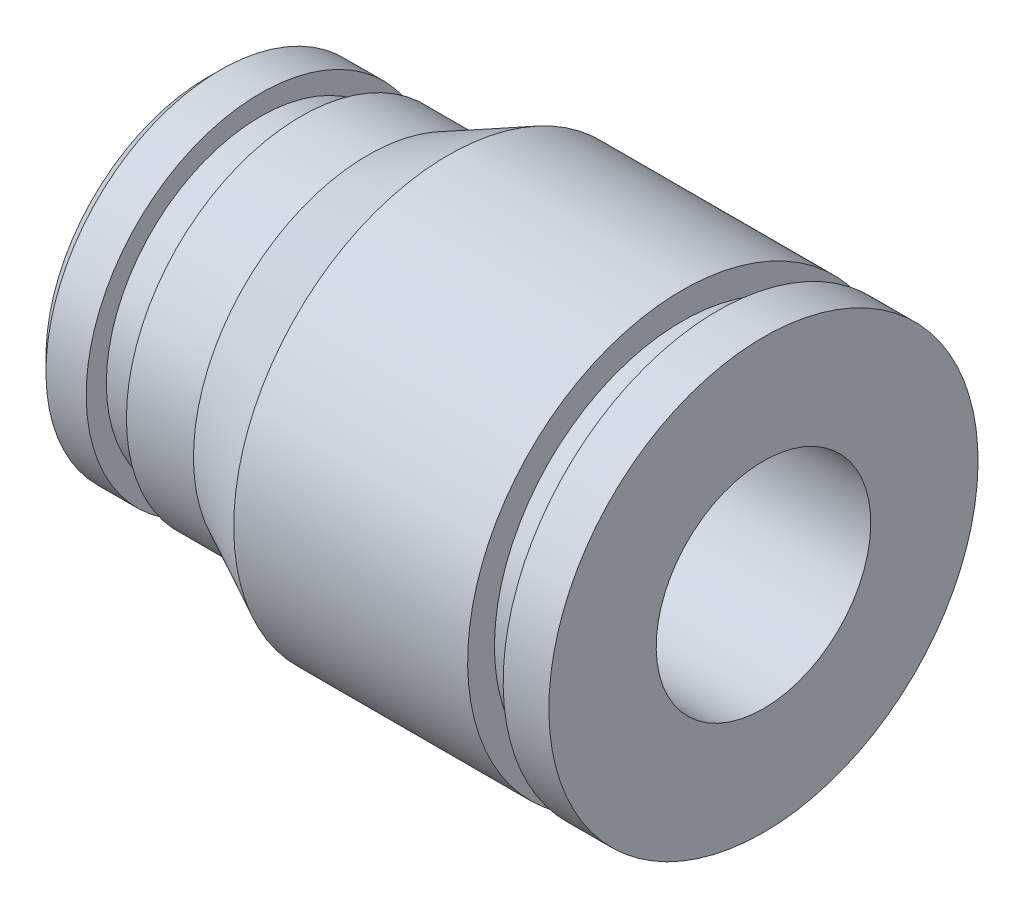
ISO-10303-21;
HEADER;
FILE_DESCRIPTION(('STEP AP214'),'2;1');
FILE_NAME('part.step','',(''),(''),'','','');
FILE_SCHEMA(('AUTOMOTIVE_DESIGN { 1 0 10303 214 1 1 1 1 }'));
ENDSEC;
DATA;
#1=APPLICATION_CONTEXT('core data for automotive mechanical design processes');
#2=APPLICATION_PROTOCOL_DEFINITION('international standard','automotive_design',2000,#1);
#3=PRODUCT_CONTEXT('',#1,'mechanical');
#4=PRODUCT('Part','Part','',(#3));
#5=PRODUCT_RELATED_PRODUCT_CATEGORY('part','',(#4));
#6=PRODUCT_DEFINITION_FORMATION('','',#4);
#7=PRODUCT_DEFINITION_CONTEXT('part definition',#1,'design');
#8=PRODUCT_DEFINITION('design','',#6,#7);
#9=PRODUCT_DEFINITION_SHAPE('','',#8);
#10=(LENGTH_UNIT() NAMED_UNIT(*) SI_UNIT(.MILLI.,.METRE.));
#11=(NAMED_UNIT(*) PLANE_ANGLE_UNIT() SI_UNIT($,.RADIAN.));
#12=(NAMED_UNIT(*) SI_UNIT($,.STERADIAN.) SOLID_ANGLE_UNIT());
#13=UNCERTAINTY_MEASURE_WITH_UNIT(LENGTH_MEASURE(1.E-05),#10,'distance_accuracy_value','');
#14=(GEOMETRIC_REPRESENTATION_CONTEXT(3) GLOBAL_UNCERTAINTY_ASSIGNED_CONTEXT((#13)) GLOBAL_UNIT_ASSIGNED_CONTEXT((#10,
#11,#12)) REPRESENTATION_CONTEXT('',''));
#15=CARTESIAN_POINT('',(0.,0.,0.));
#16=DIRECTION('',(0.,0.,1.));
#17=DIRECTION('',(1.,0.,0.));
#18=AXIS2_PLACEMENT_3D('',#15,#16,#17);
#19=CARTESIAN_POINT('',(-43.7918179780591,0.,0.));
#20=DIRECTION('',(-1.,0.,0.));
#21=DIRECTION('',(0.,-1.,0.));
#22=AXIS2_PLACEMENT_3D('',#19,#20,#21);
#23=CYLINDRICAL_SURFACE('',#22,13.);
#24=CARTESIAN_POINT('',(-8.5973527361911,0.,0.));
#25=DIRECTION('',(-1.,0.,0.));
#26=DIRECTION('',(0.,-1.,0.));
#27=AXIS2_PLACEMENT_3D('',#24,#25,#26);
#28=CIRCLE('',#27,13.);
#29=CARTESIAN_POINT('',(-8.59735273619109,-13.,0.));
#30=VERTEX_POINT('',#29);
#31=EDGE_CURVE('E76',#30,#30,#28,.T.);
#32=ORIENTED_EDGE('',*,*,#31,.F.);
#33=EDGE_LOOP('',(#32));
#34=FACE_BOUND('',#33,.T.);
#35=CARTESIAN_POINT('',(-5.59735273619109,0.,0.));
#36=DIRECTION('',(1.,0.,0.));
#37=DIRECTION('',(0.,0.,-1.));
#38=AXIS2_PLACEMENT_3D('',#35,#36,#37);
#39=CIRCLE('',#38,13.);
#40=CARTESIAN_POINT('',(-5.59735273619109,0.,-13.));
#41=VERTEX_POINT('',#40);
#42=EDGE_CURVE('E50',#41,#41,#39,.T.);
#43=ORIENTED_EDGE('',*,*,#42,.F.);
#44=EDGE_LOOP('',(#43));
#45=FACE_BOUND('',#44,.T.);
#46=ADVANCED_FACE('F43',(#34,#45),#23,.T.);
#47=CARTESIAN_POINT('',(2.4026472638089,0.,0.));
#48=DIRECTION('',(-1.,0.,0.));
#49=DIRECTION('',(0.,-1.,0.));
#50=AXIS2_PLACEMENT_3D('',#47,#48,#49);
#51=CIRCLE('',#50,13.);
#52=CARTESIAN_POINT('',(2.4026472638089,-13.,0.));
#53=VERTEX_POINT('',#52);
#54=EDGE_CURVE('E78',#53,#53,#51,.T.);
#55=ORIENTED_EDGE('',*,*,#54,.T.);
#56=EDGE_LOOP('',(#55));
#57=FACE_BOUND('',#56,.T.);
#58=CARTESIAN_POINT('',(-2.59735273619109,0.,0.));
#59=DIRECTION('',(-1.,0.,0.));
#60=DIRECTION('',(0.,0.,1.));
#61=AXIS2_PLACEMENT_3D('',#58,#59,#60);
#62=CIRCLE('',#61,13.);
#63=CARTESIAN_POINT('',(-2.59735273619109,0.,13.));
#64=VERTEX_POINT('',#63);
#65=EDGE_CURVE('E56',#64,#64,#62,.T.);
#66=ORIENTED_EDGE('',*,*,#65,.F.);
#67=EDGE_LOOP('',(#66));
#68=FACE_BOUND('',#67,.T.);
#69=ADVANCED_FACE('F115',(#57,#68),#23,.T.);
#70=CARTESIAN_POINT('',(-9.5973527361911,12.,0.));
#71=DIRECTION('',(1.,0.,0.));
#72=DIRECTION('',(0.,1.,0.));
#73=AXIS2_PLACEMENT_3D('',#70,#71,#72);
#74=PLANE('',#73);
#75=CARTESIAN_POINT('',(-9.5973527361911,0.,0.));
#76=DIRECTION('',(-1.,0.,0.));
#77=DIRECTION('',(0.,-1.,0.));
#78=AXIS2_PLACEMENT_3D('',#75,#76,#77);
#79=CIRCLE('',#78,7.99999999999999);
#80=CARTESIAN_POINT('',(-9.5973527361911,-7.99999999999999,0.));
#81=VERTEX_POINT('',#80);
#82=EDGE_CURVE('E10',#81,#81,#79,.T.);
#83=ORIENTED_EDGE('',*,*,#82,.F.);
#84=EDGE_LOOP('',(#83));
#85=FACE_BOUND('',#84,.T.);
#86=CARTESIAN_POINT('',(-9.5973527361911,0.,0.));
#87=DIRECTION('',(-1.,0.,0.));
#88=DIRECTION('',(0.,-1.,0.));
#89=AXIS2_PLACEMENT_3D('',#86,#87,#88);
#90=CIRCLE('',#89,12.);
#91=CARTESIAN_POINT('',(-9.5973527361911,-12.,0.));
#92=VERTEX_POINT('',#91);
#93=EDGE_CURVE('E64',#92,#92,#90,.T.);
#94=ORIENTED_EDGE('',*,*,#93,.T.);
#95=EDGE_LOOP('',(#94));
#96=FACE_BOUND('',#95,.T.);
#97=ADVANCED_FACE('F44',(#85,#96),#74,.F.);
#98=CARTESIAN_POINT('',(-43.7918179780591,0.,0.));
#99=DIRECTION('',(-1.,0.,0.));
#100=DIRECTION('',(0.,-1.,0.));
#101=AXIS2_PLACEMENT_3D('',#98,#99,#100);
#102=CYLINDRICAL_SURFACE('',#101,7.99999999999999);
#103=CARTESIAN_POINT('',(31.9026472638089,0.,0.));
#104=DIRECTION('',(-1.,0.,0.));
#105=DIRECTION('',(0.,-1.,0.));
#106=AXIS2_PLACEMENT_3D('',#103,#104,#105);
#107=CIRCLE('',#106,7.99999999999999);
#108=CARTESIAN_POINT('',(31.9026472638089,-7.99999999999997,0.));
#109=VERTEX_POINT('',#108);
#110=EDGE_CURVE('E51',#109,#109,#107,.T.);
#111=ORIENTED_EDGE('',*,*,#110,.F.);
#112=EDGE_LOOP('',(#111));
#113=FACE_BOUND('',#112,.T.);
#114=ORIENTED_EDGE('',*,*,#82,.T.);
#115=EDGE_LOOP('',(#114));
#116=FACE_BOUND('',#115,.T.);
#117=ADVANCED_FACE('F102',(#113,#116),#102,.F.);
#118=CARTESIAN_POINT('',(31.9026472638089,8.,0.));
#119=DIRECTION('',(-1.,0.,0.));
#120=DIRECTION('',(0.,-1.,0.));
#121=AXIS2_PLACEMENT_3D('',#118,#119,#120);
#122=PLANE('',#121);
#123=CARTESIAN_POINT('',(31.9026472638089,0.,0.));
#124=DIRECTION('',(-1.,0.,0.));
#125=DIRECTION('',(0.,-1.,0.));
#126=AXIS2_PLACEMENT_3D('',#123,#124,#125);
#127=CIRCLE('',#126,16.);
#128=CARTESIAN_POINT('',(31.9026472638089,-16.,0.));
#129=VERTEX_POINT('',#128);
#130=EDGE_CURVE('E57',#129,#129,#127,.T.);
#131=ORIENTED_EDGE('',*,*,#130,.F.);
#132=EDGE_LOOP('',(#131));
#133=FACE_BOUND('',#132,.T.);
#134=ORIENTED_EDGE('',*,*,#110,.T.);
#135=EDGE_LOOP('',(#134));
#136=FACE_BOUND('',#135,.T.);
#137=ADVANCED_FACE('F101',(#133,#136),#122,.F.);
#138=CARTESIAN_POINT('',(-43.7918179780591,0.,0.));
#139=DIRECTION('',(-1.,0.,0.));
#140=DIRECTION('',(0.,-1.,0.));
#141=AXIS2_PLACEMENT_3D('',#138,#139,#140);
#142=CYLINDRICAL_SURFACE('',#141,16.);
#143=CARTESIAN_POINT('',(28.4930543937909,0.,0.));
#144=DIRECTION('',(-1.,0.,0.));
#145=DIRECTION('',(0.,-1.,0.));
#146=AXIS2_PLACEMENT_3D('',#143,#144,#145);
#147=CIRCLE('',#146,16.);
#148=CARTESIAN_POINT('',(28.4930543937909,-16.,0.));
#149=VERTEX_POINT('',#148);
#150=EDGE_CURVE('E94',#149,#149,#147,.T.);
#151=ORIENTED_EDGE('',*,*,#150,.F.);
#152=EDGE_LOOP('',(#151));
#153=FACE_BOUND('',#152,.T.);
#154=ORIENTED_EDGE('',*,*,#130,.T.);
#155=EDGE_LOOP('',(#154));
#156=FACE_BOUND('',#155,.T.);
#157=ADVANCED_FACE('F97',(#153,#156),#142,.T.);
#158=CARTESIAN_POINT('',(28.4930543937909,16.,0.));
#159=DIRECTION('',(1.,0.,0.));
#160=DIRECTION('',(0.,1.,0.));
#161=AXIS2_PLACEMENT_3D('',#158,#159,#160);
#162=PLANE('',#161);
#163=CARTESIAN_POINT('',(28.4930543937909,0.,0.));
#164=DIRECTION('',(-1.,0.,0.));
#165=DIRECTION('',(0.,-1.,0.));
#166=AXIS2_PLACEMENT_3D('',#163,#164,#165);
#167=CIRCLE('',#166,14.);
#168=CARTESIAN_POINT('',(28.4930543937909,-14.,0.));
#169=VERTEX_POINT('',#168);
#170=EDGE_CURVE('E93',#169,#169,#167,.T.);
#171=ORIENTED_EDGE('',*,*,#170,.F.);
#172=EDGE_LOOP('',(#171));
#173=FACE_BOUND('',#172,.T.);
#174=ORIENTED_EDGE('',*,*,#150,.T.);
#175=EDGE_LOOP('',(#174));
#176=FACE_BOUND('',#175,.T.);
#177=ADVANCED_FACE('F142',(#173,#176),#162,.F.);
#178=CARTESIAN_POINT('',(-43.7918179780591,0.,0.));
#179=DIRECTION('',(-1.,0.,0.));
#180=DIRECTION('',(0.,-1.,0.));
#181=AXIS2_PLACEMENT_3D('',#178,#179,#180);
#182=CYLINDRICAL_SURFACE('',#181,14.);
#183=CARTESIAN_POINT('',(25.8438577128639,0.,0.));
#184=DIRECTION('',(-1.,0.,0.));
#185=DIRECTION('',(0.,-1.,0.));
#186=AXIS2_PLACEMENT_3D('',#183,#184,#185);
#187=CIRCLE('',#186,14.);
#188=CARTESIAN_POINT('',(25.843857712864,-14.,0.));
#189=VERTEX_POINT('',#188);
#190=EDGE_CURVE('E86',#189,#189,#187,.T.);
#191=ORIENTED_EDGE('',*,*,#190,.F.);
#192=EDGE_LOOP('',(#191));
#193=FACE_BOUND('',#192,.T.);
#194=ORIENTED_EDGE('',*,*,#170,.T.);
#195=EDGE_LOOP('',(#194));
#196=FACE_BOUND('',#195,.T.);
#197=ADVANCED_FACE('F137',(#193,#196),#182,.T.);
#198=CARTESIAN_POINT('',(25.8438577128639,14.,0.));
#199=DIRECTION('',(-1.,0.,0.));
#200=DIRECTION('',(0.,-1.,0.));
#201=AXIS2_PLACEMENT_3D('',#198,#199,#200);
#202=PLANE('',#201);
#203=CARTESIAN_POINT('',(25.8438577128639,0.,0.));
#204=DIRECTION('',(-1.,0.,0.));
#205=DIRECTION('',(0.,-1.,0.));
#206=AXIS2_PLACEMENT_3D('',#203,#204,#205);
#207=CIRCLE('',#206,16.);
#208=CARTESIAN_POINT('',(25.843857712864,-16.,0.));
#209=VERTEX_POINT('',#208);
#210=EDGE_CURVE('E84',#209,#209,#207,.T.);
#211=ORIENTED_EDGE('',*,*,#210,.F.);
#212=EDGE_LOOP('',(#211));
#213=FACE_BOUND('',#212,.T.);
#214=ORIENTED_EDGE('',*,*,#190,.T.);
#215=EDGE_LOOP('',(#214));
#216=FACE_BOUND('',#215,.T.);
#217=ADVANCED_FACE('F133',(#213,#216),#202,.F.);
#218=CARTESIAN_POINT('',(-43.7918179780591,0.,0.));
#219=DIRECTION('',(-1.,0.,0.));
#220=DIRECTION('',(0.,-1.,0.));
#221=AXIS2_PLACEMENT_3D('',#218,#219,#220);
#222=CYLINDRICAL_SURFACE('',#221,16.);
#223=CARTESIAN_POINT('',(8.40264726380891,0.,0.));
#224=DIRECTION('',(-1.,0.,0.));
#225=DIRECTION('',(0.,-1.,0.));
#226=AXIS2_PLACEMENT_3D('',#223,#224,#225);
#227=CIRCLE('',#226,16.);
#228=CARTESIAN_POINT('',(8.40264726380891,-16.,0.));
#229=VERTEX_POINT('',#228);
#230=EDGE_CURVE('E85',#229,#229,#227,.T.);
#231=ORIENTED_EDGE('',*,*,#230,.F.);
#232=EDGE_LOOP('',(#231));
#233=FACE_BOUND('',#232,.T.);
#234=ORIENTED_EDGE('',*,*,#210,.T.);
#235=EDGE_LOOP('',(#234));
#236=FACE_BOUND('',#235,.T.);
#237=ADVANCED_FACE('F128',(#233,#236),#222,.T.);
#238=CARTESIAN_POINT('',(8.40264726380891,0.,0.));
#239=DIRECTION('',(1.,0.,0.));
#240=DIRECTION('',(0.,1.,0.));
#241=AXIS2_PLACEMENT_3D('',#238,#239,#240);
#242=CONICAL_SURFACE('',#241,16.,0.463647609000805);
#243=ORIENTED_EDGE('',*,*,#54,.F.);
#244=EDGE_LOOP('',(#243));
#245=FACE_BOUND('',#244,.T.);
#246=ORIENTED_EDGE('',*,*,#230,.T.);
#247=EDGE_LOOP('',(#246));
#248=FACE_BOUND('',#247,.T.);
#249=ADVANCED_FACE('F130',(#245,#248),#242,.T.);
#250=CARTESIAN_POINT('',(-8.5973527361911,0.,0.));
#251=DIRECTION('',(1.,0.,0.));
#252=DIRECTION('',(0.,1.,0.));
#253=AXIS2_PLACEMENT_3D('',#250,#251,#252);
#254=CONICAL_SURFACE('',#253,13.,0.785398163397448);
#255=ORIENTED_EDGE('',*,*,#93,.F.);
#256=EDGE_LOOP('',(#255));
#257=FACE_BOUND('',#256,.T.);
#258=ORIENTED_EDGE('',*,*,#31,.T.);
#259=EDGE_LOOP('',(#258));
#260=FACE_BOUND('',#259,.T.);
#261=ADVANCED_FACE('F124',(#257,#260),#254,.T.);
#262=CARTESIAN_POINT('',(-5.59735273619109,15.5441022054915,0.));
#263=DIRECTION('',(1.,0.,0.));
#264=DIRECTION('',(0.,0.,-1.));
#265=AXIS2_PLACEMENT_3D('',#262,#263,#264);
#266=PLANE('',#265);
#267=CARTESIAN_POINT('',(-5.59735273619109,0.,0.));
#268=DIRECTION('',(-1.,0.,0.));
#269=DIRECTION('',(0.,0.,1.));
#270=AXIS2_PLACEMENT_3D('',#267,#268,#269);
#271=CIRCLE('',#270,11.4980941945004);
#272=CARTESIAN_POINT('',(-5.59735273619109,0.,11.4980941945004));
#273=VERTEX_POINT('',#272);
#274=EDGE_CURVE('E61',#273,#273,#271,.T.);
#275=ORIENTED_EDGE('',*,*,#274,.T.);
#276=EDGE_LOOP('',(#275));
#277=FACE_BOUND('',#276,.T.);
#278=ORIENTED_EDGE('',*,*,#42,.T.);
#279=EDGE_LOOP('',(#278));
#280=FACE_BOUND('',#279,.T.);
#281=ADVANCED_FACE('F182',(#277,#280),#266,.T.);
#282=CARTESIAN_POINT('',(-2.5973527361911,15.5441022054915,0.));
#283=DIRECTION('',(-1.,0.,0.));
#284=DIRECTION('',(0.,0.,1.));
#285=AXIS2_PLACEMENT_3D('',#282,#283,#284);
#286=PLANE('',#285);
#287=CARTESIAN_POINT('',(-2.5973527361911,0.,0.));
#288=DIRECTION('',(-1.,0.,0.));
#289=DIRECTION('',(0.,0.,1.));
#290=AXIS2_PLACEMENT_3D('',#287,#288,#289);
#291=CIRCLE('',#290,11.4980941945004);
#292=CARTESIAN_POINT('',(-2.5973527361911,0.,11.4980941945004));
#293=VERTEX_POINT('',#292);
#294=EDGE_CURVE('E70',#293,#293,#291,.T.);
#295=ORIENTED_EDGE('',*,*,#294,.F.);
#296=EDGE_LOOP('',(#295));
#297=FACE_BOUND('',#296,.T.);
#298=ORIENTED_EDGE('',*,*,#65,.T.);
#299=EDGE_LOOP('',(#298));
#300=FACE_BOUND('',#299,.T.);
#301=ADVANCED_FACE('F187',(#297,#300),#286,.T.);
#302=CARTESIAN_POINT('',(-18.3977330245028,0.,0.));
#303=DIRECTION('',(-1.,0.,0.));
#304=DIRECTION('',(0.,0.,1.));
#305=AXIS2_PLACEMENT_3D('',#302,#303,#304);
#306=CYLINDRICAL_SURFACE('',#305,11.4980941945004);
#307=ORIENTED_EDGE('',*,*,#294,.T.);
#308=EDGE_LOOP('',(#307));
#309=FACE_BOUND('',#308,.T.);
#310=ORIENTED_EDGE('',*,*,#274,.F.);
#311=EDGE_LOOP('',(#310));
#312=FACE_BOUND('',#311,.T.);
#313=ADVANCED_FACE('F193',(#309,#312),#306,.T.);
#314=CLOSED_SHELL('',(#46,#69,#97,#117,#137,#157,#177,#197,#217,#237,#249,#261,#281,#301,#313));
#315=MANIFOLD_SOLID_BREP('B2',#314);
#316=ADVANCED_BREP_SHAPE_REPRESENTATION('',(#18,#315),#14);
#317=SHAPE_DEFINITION_REPRESENTATION(#9,#316);
ENDSEC;
END-ISO-10303-21;
